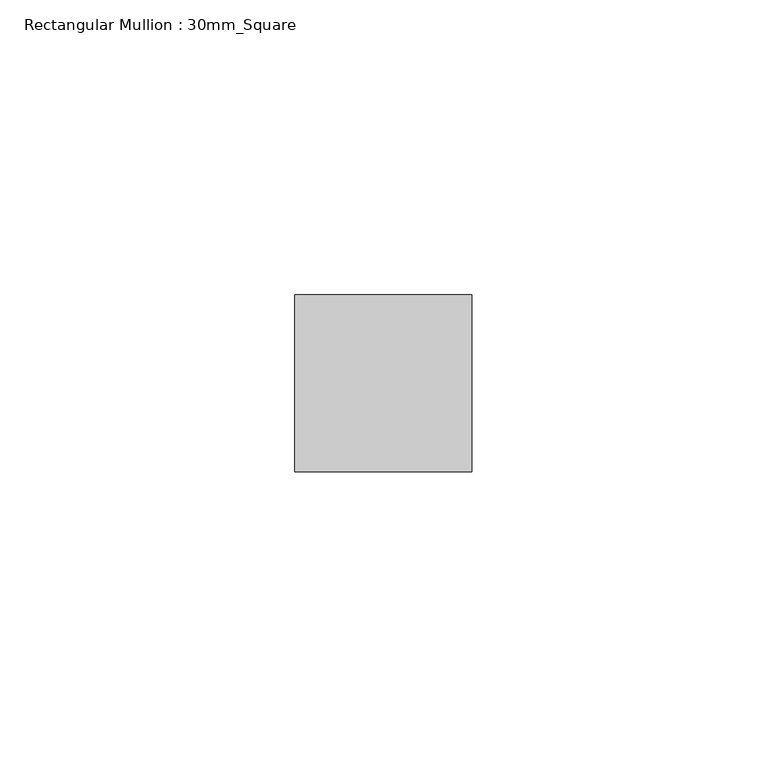
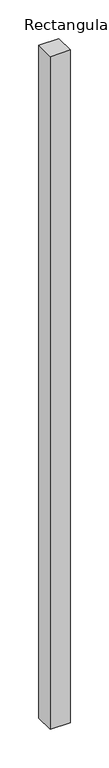
"""IFC4 building model written with IfcOpenShell, lengths in millimetres: member geometry, Rectangular Mullion : 30mm_Square."""

from ifc_helpers import new_model, si_unit, frame, origin, place, context, project, spatial, polyline, outline, extrude, source, transform, mapped, element, save


def rectangular_mullion_30mm_square_8997babb(model_context):
    return source(origin(), model_context, "Body", "SweptSolid", [
        extrude(outline(polyline([(15.0, 15.0), (15.0, -15.0), (-15.0, -15.0), (-15.0, 15.0), (15.0, 15.0)])), frame((0.0, 0.0, -1066.8), z_axis=(0.0, 0.0, 1.0), x_axis=(1.0, 0.0, 0.0)), (0.0, 0.0, 1.0), 1066.8),
    ])


if __name__ == "__main__":
    model = new_model("IFC4")
    model_context = context("Model", 3, world=origin())
    ifc_project = project(units=[si_unit("LENGTHUNIT", "METRE", prefix="MILLI")], contexts=[model_context])
    site = spatial("IfcSite", under=ifc_project)
    building = spatial("IfcBuilding", under=site)
    placement = place(None, origin())
    rectangular_mullion_30mm_square_shape = rectangular_mullion_30mm_square_8997babb(model_context)
    element("IfcMember", 1, ObjectType="Rectangular Mullion : 30mm_Square", at=placement, inside=building, context=model_context, shape_type="MappedRepresentation", body=[
        mapped(rectangular_mullion_30mm_square_shape, transform((0.0, 0.0, 0.0), x_axis=(1.0, 0.0, 0.0), y_axis=(0.0, 1.0, 0.0), z_axis=(0.0, 0.0, 1.0))),
    ])
    save(model, "model.ifc")

# Revit data of these elements
# Type "Rectangular Mullion : 30mm_Square"
#   Keynote = "H11"
#   built-in parameter 1007304 = 0.0984252 (stored number, unit not read)
#   built-in parameter 1007301 = 0.0492126 (stored number, unit not read)
#   built-in parameter 1007300 = 0.0492126 (stored number, unit not read)
# Element 1 (IfcMember, "Rectangular Mullion : 30mm_Square")
#   Materials on its faces: "Aluminium"
# Materials
#   "Aluminium": class "Metal", colour RGB 247 247 247, transparency 0, Description = "Aluminium 6061", Cost = 0
